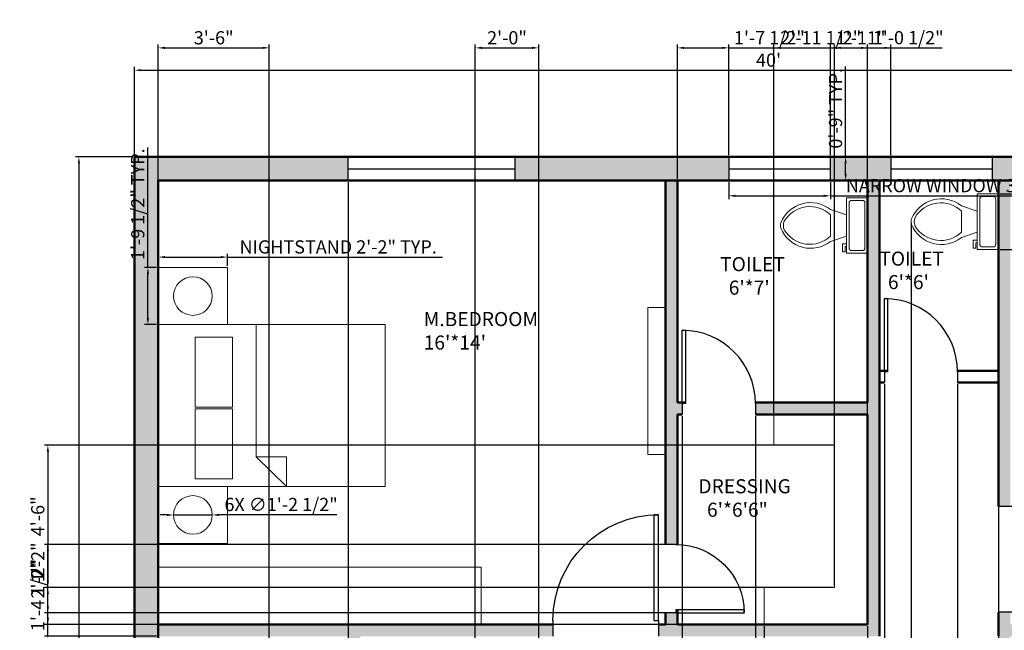
# Model space of a CAD drawing. Units: inches. Extents: x 2152 to 2718, y 1095 to 1798.
# Tile 4 of 5: x 2152 to 2524, y 1567 to 1798. Entities that reach past the tile are written whole.
import ezdxf

# ---------------------------------------------------------------- set-up
doc = ezdxf.new("R2010")
doc.units = ezdxf.units.IN
for name, color, linetype, lineweight in [('A-ANNO-DIMS', 130, 'Continuous', 18), ('A-AREA-IDEN', 130, 'Continuous', 25), ('A-FLOR-CASE', 10, 'Continuous', 20), ('A-FLOR-FIXT', 10, 'Continuous', 18), ('A-WALL-PATT', 210, 'Continuous', 13), ('DOOR', 160, 'Continuous', 25), ('FUR', 10, 'Continuous', 18), ('WALL', 7, 'Continuous', 50), ('WIND', 140, 'Continuous', 25)]:
    doc.layers.add(name, color=color, linetype=linetype, lineweight=lineweight)
doc.styles.get("Standard").update_dxf_attribs({"font": 'arial.ttf'})
doc.dimstyles.new('ISO-25', dxfattribs={"dimtxt": 5, "dimasz": 2.5, "dimexe": 1.25, "dimexo": 0.625, "dimtad": 1, "dimdec": 0, "dimlunit": 4, "dimtxsty": 'Standard', "dimcen": 2.5, "dimadec": 0, "dimazin": 0, "dimtfac": 1, "dimtdec": 0, "dimtmove": 0, "dimatfit": 3, "dimfxl": 1, "dimarcsym": 0})

# ---------------------------------------------------------------- blocks, each defined once
blk = doc.blocks.new('*U2')
for p, q in [((0, 0), (0, -6)), ((40, 0), (40, -6))]:
    blk.add_line(p, q)
blk.add_lwpolyline([(0, 0), (0, 40), (1.75, 40), (1.75, 0)], close=True)
blk.add_arc((0, 0), 40, 0, 90)
blk = doc.blocks.new('*U8')
for p, q in [((9.5, -6), (9.5, -2)), ((-10, -8.5), (-8, -8.5)), ((-10, -9.5), (-10, -8.5)), ((-7, -9.5), (-10, -9.5)), ((-8, -8.5), (-8, -8)), ((-7, -8), (-7, -9.5)), ((-4, -8), (-6, -14)), ((4, -8), (6, -14)), ((4, -14), (-4, -14))]:
    blk.add_line(p, q)
blk.add_lwpolyline([(10.5, -8), (10.5, 0), (-10.5, 0), (-10.5, -8)], close=True)
for points in [[(-9.5, -2), (-9.5, -6)], [(8.5, -1), (-8.5, -1)], [(-8.5, -7), (8.5, -7)]]:
    blk.add_lwpolyline(points)
for centre, radius, start, end in [((-8.62, -1.88), 0.884, 81.8699, 188.1301), ((8.62, -1.88), 0.884, 351.8699, 98.1301), ((-8.62, -6.12), 0.884, 171.8699, 278.1301), ((8.62, -6.12), 0.884, 261.8699, 8.1301), ((3.52, -21.58), 12.17, 141.4691, 247.9714), ((4.2, -21.82), 11.33, 136.3677, 238.9468), ((-3.52, -21.58), 12.17, 292.0284, 38.5307), ((-4.2, -21.82), 11.33, 301.053, 43.6321), ((0, -27.88), 4, 245.7318, 294.2682), ((0, -29), 4, 254.8605, 285.1395)]:
    blk.add_arc(centre, radius, start, end)
blk = doc.blocks.new('*D13')
at = {"layer": 'A-ANNO-DIMS', "color": 0, "lineweight": -2, "transparency": 16777216}
for p, q in [((2195.06, 1746.99), (2195.06, 1780.4)), ((2197.56, 1779.15), (2672.56, 1779.15)), ((2675.06, 1746.99), (2675.06, 1780.4))]:
    blk.add_line(p, q, dxfattribs=at)
at = {"layer": 'A-ANNO-DIMS', "color": 0, "transparency": 16777216}
for points in [[(2197.56, 1779.57), (2197.56, 1778.74), (2195.06, 1779.15)], [(2672.56, 1779.57), (2672.56, 1778.74), (2675.06, 1779.15)]]:
    blk.add_solid(points, dxfattribs=at)
at = {"layer": 'Defpoints', "color": 0, "transparency": 16777216}
for p in [(2675.06, 1779.15), (2195.06, 1746.37), (2675.06, 1746.37)]:
    blk.add_point(p, dxfattribs=at)
at = {"layer": 'A-ANNO-DIMS', "color": 0, "transparency": 16777216, "insert": (2435.06, 1782.33), "char_height": 5, "attachment_point": 5}
blk.add_mtext("40'", dxfattribs=at)
blk = doc.blocks.new('*D14')
at = {"layer": 'A-ANNO-DIMS', "color": 0, "lineweight": -2, "transparency": 16777216}
for p, q in [((2194.43, 1746.37), (2172.77, 1746.37)), ((2174.02, 1743.87), (2174.02, 1136.72)), ((2194.43, 1134.22), (2172.77, 1134.22))]:
    blk.add_line(p, q, dxfattribs=at)
at = {"layer": 'A-ANNO-DIMS', "color": 0, "transparency": 16777216}
for points in [[(2173.6, 1743.87), (2174.43, 1743.87), (2174.02, 1746.37)], [(2173.6, 1136.72), (2174.43, 1136.72), (2174.02, 1134.22)]]:
    blk.add_solid(points, dxfattribs=at)
at = {"layer": 'Defpoints', "color": 0, "transparency": 16777216}
for p in [(2195.06, 1746.37), (2174.02, 1134.22), (2195.06, 1134.22)]:
    blk.add_point(p, dxfattribs=at)
at = {"layer": 'A-ANNO-DIMS', "color": 0, "transparency": 16777216, "insert": (2170.84, 1440.29), "char_height": 5, "attachment_point": 5, "rotation": 90}
blk.add_mtext("51'", dxfattribs=at)
blk = doc.blocks.new('WIN-WIDE')
blk.add_line((0, 4.5), (63.07, 4.5))
blk.add_lwpolyline([(0, 9), (63.07, 9), (63.07, 0), (0, 0)], close=True)
blk = doc.blocks.new('WIN-NARROW')
blk.add_line((0, 4.5), (38.45, 4.5))
blk.add_lwpolyline([(0, 0), (38.45, 0), (38.45, 9), (0, 9)], close=True)
blk = doc.blocks.new('BED-DOUBLE')
for p, q in [((37.05, 61.24), (37.05, 11.23)), ((37.05, 11.23), (48.59, 11.23)), ((48.59, 0), (37.05, 11.23)), ((48.59, 11.23), (48.59, 0))]:
    blk.add_line(p, q)
for points in [[(0, 61.24), (85.82, 61.24), (85.82, 0), (0, 0)], [(13.94, 29.93), (28.11, 29.93), (28.11, 56.53), (13.94, 56.53)], [(13.94, 2.81), (28.11, 2.81), (28.11, 29.41), (13.94, 29.41)]]:
    blk.add_lwpolyline(points, close=True)
blk = doc.blocks.new('NIGHTSTAND')
blk.add_lwpolyline([(0, 21.63), (26.19, 21.63), (26.19, 0), (0, 0)], close=True)
blk.add_circle((13.1, 10.82), 7.32)
blk = doc.blocks.new('*D22')
at = {"layer": 'A-ANNO-DIMS', "color": 0, "lineweight": -2, "transparency": 16777216}
for p, q in [((2204.06, 1705.1), (2204.06, 1709.65)), ((2206.56, 1708.4), (2227.75, 1708.4)), ((2230.25, 1705.1), (2230.25, 1709.65)), ((2230.25, 1708.4), (2311.58, 1708.4))]:
    blk.add_line(p, q, dxfattribs=at)
at = {"layer": 'A-ANNO-DIMS', "color": 0, "transparency": 16777216}
for points in [[(2206.56, 1708.82), (2206.56, 1707.99), (2204.06, 1708.4)], [(2227.75, 1708.82), (2227.75, 1707.99), (2230.25, 1708.4)]]:
    blk.add_solid(points, dxfattribs=at)
at = {"layer": 'Defpoints', "color": 0, "transparency": 16777216}
for p in [(2230.25, 1708.4), (2204.06, 1704.48), (2230.25, 1704.48)]:
    blk.add_point(p, dxfattribs=at)
at = {"layer": 'A-ANNO-DIMS', "color": 0, "transparency": 16777216, "insert": (2272.16, 1711.61), "char_height": 5, "attachment_point": 5}
blk.add_mtext('NIGHTSTAND 2\'-2" TYP.', dxfattribs=at)
blk = doc.blocks.new('*D23')
at = {"layer": 'A-ANNO-DIMS', "color": 0, "lineweight": -2, "transparency": 16777216}
for p, q in [((2200.13, 1704.48), (2200.13, 1749.88)), ((2203.43, 1704.48), (2198.88, 1704.48)), ((2200.13, 1685.34), (2200.13, 1701.98)), ((2203.43, 1682.84), (2198.88, 1682.84))]:
    blk.add_line(p, q, dxfattribs=at)
at = {"layer": 'A-ANNO-DIMS', "color": 0, "transparency": 16777216}
for points in [[(2199.71, 1701.98), (2200.55, 1701.98), (2200.13, 1704.48)], [(2199.71, 1685.34), (2200.55, 1685.34), (2200.13, 1682.84)]]:
    blk.add_solid(points, dxfattribs=at)
at = {"layer": 'Defpoints', "color": 0, "transparency": 16777216}
for p in [(2200.13, 1704.48), (2204.06, 1704.48), (2204.06, 1682.84)]:
    blk.add_point(p, dxfattribs=at)
at = {"layer": 'A-ANNO-DIMS', "color": 0, "transparency": 16777216, "insert": (2196.92, 1728.43), "char_height": 5, "attachment_point": 5, "rotation": 90}
blk.add_mtext('1\'-9 1/2" TYP.', dxfattribs=at)
blk = doc.blocks.new('*D26')
at = {"layer": 'A-ANNO-DIMS', "color": 0, "lineweight": -2, "transparency": 16777216}
for p, q in [((2420.03, 1736.74), (2420.03, 1730.35)), ((2458.48, 1736.74), (2458.48, 1730.35)), ((2422.53, 1731.6), (2455.98, 1731.6)), ((2458.48, 1731.6), (2570.46, 1731.6))]:
    blk.add_line(p, q, dxfattribs=at)
at = {"layer": 'A-ANNO-DIMS', "color": 0, "transparency": 16777216}
for points in [[(2422.53, 1732.02), (2422.53, 1731.18), (2420.03, 1731.6)], [(2455.98, 1732.02), (2455.98, 1731.18), (2458.48, 1731.6)]]:
    blk.add_solid(points, dxfattribs=at)
at = {"layer": 'Defpoints', "color": 0, "transparency": 16777216}
for p in [(2420.03, 1737.37), (2458.48, 1737.37), (2458.48, 1731.6)]:
    blk.add_point(p, dxfattribs=at)
at = {"layer": 'A-ANNO-DIMS', "color": 0, "transparency": 16777216, "insert": (2515.72, 1734.81), "char_height": 5, "attachment_point": 5}
blk.add_mtext('NARROW WINDOW 3\'-2 1/2" TYP.', dxfattribs=at)
blk = doc.blocks.new('*D27')
at = {"layer": 'A-ANNO-DIMS', "color": 0, "lineweight": -2, "transparency": 16777216}
for p, q in [((2464.24, 1746.37), (2464.24, 1780.59)), ((2459.1, 1746.37), (2465.49, 1746.37)), ((2464.24, 1739.87), (2464.24, 1743.87)), ((2459.1, 1737.37), (2465.49, 1737.37))]:
    blk.add_line(p, q, dxfattribs=at)
at = {"layer": 'A-ANNO-DIMS', "color": 0, "transparency": 16777216}
for points in [[(2463.83, 1743.87), (2464.66, 1743.87), (2464.24, 1746.37)], [(2463.83, 1739.87), (2464.66, 1739.87), (2464.24, 1737.37)]]:
    blk.add_solid(points, dxfattribs=at)
at = {"layer": 'Defpoints', "color": 0, "transparency": 16777216}
for p in [(2458.48, 1746.37), (2464.24, 1746.37), (2458.48, 1737.37)]:
    blk.add_point(p, dxfattribs=at)
at = {"layer": 'A-ANNO-DIMS', "color": 0, "transparency": 16777216, "insert": (2461.07, 1764.73), "char_height": 5, "attachment_point": 5, "rotation": 90}
blk.add_mtext('0\'-9" TYP.', dxfattribs=at)
blk = doc.blocks.new('*D36')
at = {"layer": 'A-ANNO-DIMS', "color": 0, "lineweight": -2, "transparency": 16777216}
for p, q in [((2204.06, 1736.74), (2204.06, 1098.09)), ((2275.93, 1736.74), (2275.93, 1098.09)), ((2206.56, 1099.34), (2273.43, 1099.34))]:
    blk.add_line(p, q, dxfattribs=at)
at = {"layer": 'A-ANNO-DIMS', "color": 0, "transparency": 16777216}
for points in [[(2206.56, 1099.75), (2206.56, 1098.92), (2204.06, 1099.34)], [(2273.43, 1099.75), (2273.43, 1098.92), (2275.93, 1099.34)]]:
    blk.add_solid(points, dxfattribs=at)
at = {"layer": 'Defpoints', "color": 0, "transparency": 16777216}
for p in [(2204.06, 1737.37), (2275.93, 1737.37), (2275.93, 1099.34)]:
    blk.add_point(p, dxfattribs=at)
at = {"layer": 'A-ANNO-DIMS', "color": 0, "transparency": 16777216, "insert": (2240, 1102.51), "char_height": 5, "attachment_point": 5}
blk.add_mtext('6\'-0"', dxfattribs=at)
blk = doc.blocks.new('*D37')
at = {"layer": 'A-ANNO-DIMS', "color": 0, "lineweight": -2, "transparency": 16777216}
for p, q in [((2400.56, 1737.99), (2400.56, 1788.86)), ((2403.06, 1787.61), (2417.53, 1787.61)), ((2420.03, 1746.99), (2420.03, 1788.86)), ((2420.03, 1787.61), (2448.25, 1787.61))]:
    blk.add_line(p, q, dxfattribs=at)
at = {"layer": 'A-ANNO-DIMS', "color": 0, "transparency": 16777216}
for points in [[(2403.06, 1788.03), (2403.06, 1787.19), (2400.56, 1787.61)], [(2417.53, 1788.03), (2417.53, 1787.19), (2420.03, 1787.61)]]:
    blk.add_solid(points, dxfattribs=at)
at = {"layer": 'Defpoints', "color": 0, "transparency": 16777216}
for p in [(2420.03, 1787.61), (2420.03, 1746.37), (2400.56, 1737.37)]:
    blk.add_point(p, dxfattribs=at)
at = {"layer": 'A-ANNO-DIMS', "color": 0, "transparency": 16777216, "insert": (2435.39, 1790.82), "char_height": 5, "attachment_point": 5}
blk.add_mtext('1\'-7 1/2"', dxfattribs=at)
blk = doc.blocks.new('*D38')
at = {"layer": 'A-ANNO-DIMS', "color": 0, "lineweight": -2, "transparency": 16777216}
for p, q in [((2458.48, 1746.99), (2458.48, 1788.86)), ((2460.98, 1787.61), (2478.85, 1787.61)), ((2481.35, 1746.99), (2481.35, 1788.86))]:
    blk.add_line(p, q, dxfattribs=at)
at = {"layer": 'A-ANNO-DIMS', "color": 0, "transparency": 16777216}
for points in [[(2460.98, 1788.03), (2460.98, 1787.19), (2458.48, 1787.61)], [(2478.85, 1788.03), (2478.85, 1787.19), (2481.35, 1787.61)]]:
    blk.add_solid(points, dxfattribs=at)
at = {"layer": 'Defpoints', "color": 0, "transparency": 16777216}
for p in [(2481.35, 1787.61), (2458.48, 1746.37), (2481.35, 1746.37)]:
    blk.add_point(p, dxfattribs=at)
at = {"layer": 'A-ANNO-DIMS', "color": 0, "transparency": 16777216, "insert": (2469.91, 1790.75), "char_height": 5, "attachment_point": 5}
blk.add_mtext('1\'-11"', dxfattribs=at)
blk = doc.blocks.new('*D40')
at = {"layer": 'A-ANNO-DIMS', "color": 0, "lineweight": -2, "transparency": 16777216}
for p, q in [((2162.26, 1564.87), (2162.26, 1593.09)), ((2203.43, 1564.87), (2161.01, 1564.87)), ((2162.26, 1550.66), (2162.26, 1562.37)), ((2203.43, 1548.16), (2161.01, 1548.16))]:
    blk.add_line(p, q, dxfattribs=at)
at = {"layer": 'A-ANNO-DIMS', "color": 0, "transparency": 16777216}
for points in [[(2161.84, 1562.37), (2162.68, 1562.37), (2162.26, 1564.87)], [(2161.84, 1550.66), (2162.68, 1550.66), (2162.26, 1548.16)]]:
    blk.add_solid(points, dxfattribs=at)
at = {"layer": 'Defpoints', "color": 0, "transparency": 16777216}
for p in [(2162.26, 1564.87), (2204.06, 1564.87), (2204.06, 1548.16)]:
    blk.add_point(p, dxfattribs=at)
at = {"layer": 'A-ANNO-DIMS', "color": 0, "transparency": 16777216, "insert": (2159.05, 1580.23), "char_height": 5, "attachment_point": 5, "rotation": 90}
blk.add_mtext('1\'-4 1/2"', dxfattribs=at)
blk = doc.blocks.new('*D42')
at = {"layer": 'A-ANNO-DIMS', "color": 0, "lineweight": -2, "transparency": 16777216}
for p, q in [((2204.06, 1176.99), (2204.06, 1788.86)), ((2206.56, 1787.61), (2243.52, 1787.61)), ((2246.02, 1176.99), (2246.02, 1788.86))]:
    blk.add_line(p, q, dxfattribs=at)
at = {"layer": 'A-ANNO-DIMS', "color": 0, "transparency": 16777216}
for points in [[(2206.56, 1788.03), (2206.56, 1787.19), (2204.06, 1787.61)], [(2243.52, 1788.03), (2243.52, 1787.19), (2246.02, 1787.61)]]:
    blk.add_solid(points, dxfattribs=at)
at = {"layer": 'Defpoints', "color": 0, "transparency": 16777216}
for p in [(2246.02, 1787.61), (2204.06, 1176.37), (2246.02, 1176.37)]:
    blk.add_point(p, dxfattribs=at)
at = {"layer": 'A-ANNO-DIMS', "color": 0, "transparency": 16777216, "insert": (2225.04, 1790.79), "char_height": 5, "attachment_point": 5}
blk.add_mtext('3\'-6"', dxfattribs=at)
blk = doc.blocks.new('*D50')
at = {"layer": 'A-ANNO-DIMS', "color": 0, "lineweight": -2, "transparency": 16777216}
for p, q in [((2707.86, 1560.98), (2707.86, 1589.76)), ((2281.18, 1560.98), (2709.11, 1560.98)), ((2707.86, 1539.09), (2707.86, 1558.48)), ((2281.18, 1536.59), (2709.11, 1536.59))]:
    blk.add_line(p, q, dxfattribs=at)
at = {"layer": 'A-ANNO-DIMS', "color": 0, "transparency": 16777216}
for points in [[(2707.44, 1558.48), (2708.28, 1558.48), (2707.86, 1560.98)], [(2707.44, 1539.09), (2708.28, 1539.09), (2707.86, 1536.59)]]:
    blk.add_solid(points, dxfattribs=at)
at = {"layer": 'Defpoints', "color": 0, "transparency": 16777216}
for p in [(2280.56, 1560.98), (2707.86, 1560.98), (2280.56, 1536.59)]:
    blk.add_point(p, dxfattribs=at)
at = {"layer": 'A-ANNO-DIMS', "color": 0, "transparency": 16777216, "insert": (2704.65, 1576.62), "char_height": 5, "attachment_point": 5, "rotation": 90}
blk.add_mtext('2\'-0 1/2"', dxfattribs=at)
blk = doc.blocks.new('*D51')
at = {"layer": 'A-ANNO-DIMS', "color": 0, "lineweight": -2, "transparency": 16777216}
for p, q in [((2399.93, 1599.6), (2161.01, 1599.6)), ((2162.26, 1576.22), (2162.26, 1597.1)), ((2399.32, 1573.72), (2161.01, 1573.72))]:
    blk.add_line(p, q, dxfattribs=at)
at = {"layer": 'A-ANNO-DIMS', "color": 0, "transparency": 16777216}
for points in [[(2161.84, 1597.1), (2162.68, 1597.1), (2162.26, 1599.6)], [(2161.84, 1576.22), (2162.68, 1576.22), (2162.26, 1573.72)]]:
    blk.add_solid(points, dxfattribs=at)
at = {"layer": 'Defpoints', "color": 0, "transparency": 16777216}
for p in [(2162.26, 1599.6), (2400.56, 1599.6), (2399.94, 1573.72)]:
    blk.add_point(p, dxfattribs=at)
at = {"layer": 'A-ANNO-DIMS', "color": 0, "transparency": 16777216, "insert": (2159.12, 1586.66), "char_height": 5, "attachment_point": 5, "rotation": 90}
blk.add_mtext('2\'-2"', dxfattribs=at)
blk = doc.blocks.new('*D52')
at = {"layer": 'A-ANNO-DIMS', "color": 0, "lineweight": -2, "transparency": 16777216}
for p, q in [((2402.42, 1648.24), (2402.42, 1098.09)), ((2430.09, 1648.24), (2430.09, 1098.09)), ((2404.92, 1099.34), (2427.59, 1099.34))]:
    blk.add_line(p, q, dxfattribs=at)
at = {"layer": 'A-ANNO-DIMS', "color": 0, "transparency": 16777216}
for points in [[(2404.92, 1099.75), (2404.92, 1098.92), (2402.42, 1099.34)], [(2427.59, 1099.75), (2427.59, 1098.92), (2430.09, 1099.34)]]:
    blk.add_solid(points, dxfattribs=at)
at = {"layer": 'Defpoints', "color": 0, "transparency": 16777216}
for p in [(2402.42, 1648.87), (2430.09, 1648.87), (2430.09, 1099.34)]:
    blk.add_point(p, dxfattribs=at)
at = {"layer": 'A-ANNO-DIMS', "color": 0, "transparency": 16777216, "insert": (2416.26, 1102.55), "char_height": 5, "attachment_point": 5}
blk.add_mtext('2\'-3 1/2"', dxfattribs=at)
blk = doc.blocks.new('*D57')
at = {"layer": 'A-ANNO-DIMS', "color": 0, "lineweight": -2, "transparency": 16777216}
for p, q in [((2489.06, 1721.19), (2489.06, 1098.09)), ((2522.06, 1710.69), (2522.06, 1098.09)), ((2491.56, 1099.34), (2519.56, 1099.34))]:
    blk.add_line(p, q, dxfattribs=at)
at = {"layer": 'A-ANNO-DIMS', "color": 0, "transparency": 16777216}
for points in [[(2491.56, 1099.75), (2491.56, 1098.92), (2489.06, 1099.34)], [(2519.56, 1099.75), (2519.56, 1098.92), (2522.06, 1099.34)]]:
    blk.add_solid(points, dxfattribs=at)
at = {"layer": 'Defpoints', "color": 0, "transparency": 16777216}
for p in [(2489.06, 1721.81), (2522.06, 1711.31), (2522.06, 1099.34)]:
    blk.add_point(p, dxfattribs=at)
at = {"layer": 'A-ANNO-DIMS', "color": 0, "transparency": 16777216, "insert": (2505.56, 1102.51), "char_height": 5, "attachment_point": 5}
blk.add_mtext('2\'-9"', dxfattribs=at)
blk = doc.blocks.new('*D58')
at = {"layer": 'A-ANNO-DIMS', "color": 0, "lineweight": -2, "transparency": 16777216}
for p, q in [((2522.68, 1732.31), (2709.11, 1732.31)), ((2707.86, 1729.81), (2707.86, 1713.81)), ((2522.68, 1711.31), (2709.11, 1711.31))]:
    blk.add_line(p, q, dxfattribs=at)
at = {"layer": 'A-ANNO-DIMS', "color": 0, "transparency": 16777216}
for points in [[(2707.44, 1729.81), (2708.28, 1729.81), (2707.86, 1732.31)], [(2707.44, 1713.81), (2708.28, 1713.81), (2707.86, 1711.31)]]:
    blk.add_solid(points, dxfattribs=at)
at = {"layer": 'Defpoints', "color": 0, "transparency": 16777216}
for p in [(2522.06, 1732.31), (2522.06, 1711.31), (2707.86, 1711.31)]:
    blk.add_point(p, dxfattribs=at)
at = {"layer": 'A-ANNO-DIMS', "color": 0, "transparency": 16777216, "insert": (2704.68, 1721.81), "char_height": 5, "attachment_point": 5, "rotation": 90}
blk.add_mtext('1\'-9"', dxfattribs=at)
blk = doc.blocks.new('*D59')
at = {"layer": 'A-ANNO-DIMS', "color": 0, "lineweight": -2, "transparency": 16777216}
for p, q in [((2478.92, 1660.24), (2478.92, 1098.09)), ((2506.58, 1660.24), (2506.58, 1098.09)), ((2481.42, 1099.34), (2504.08, 1099.34))]:
    blk.add_line(p, q, dxfattribs=at)
at = {"layer": 'A-ANNO-DIMS', "color": 0, "transparency": 16777216}
for points in [[(2481.42, 1099.75), (2481.42, 1098.92), (2478.92, 1099.34)], [(2504.08, 1099.75), (2504.08, 1098.92), (2506.58, 1099.34)]]:
    blk.add_solid(points, dxfattribs=at)
at = {"layer": 'Defpoints', "color": 0, "transparency": 16777216}
for p in [(2478.92, 1660.87), (2506.58, 1660.87), (2506.58, 1099.34)]:
    blk.add_point(p, dxfattribs=at)
at = {"layer": 'A-ANNO-DIMS', "color": 0, "transparency": 16777216, "insert": (2492.75, 1102.55), "char_height": 5, "attachment_point": 5}
blk.add_mtext('2\'-3 1/2"', dxfattribs=at)
blk = doc.blocks.new('*D60')
at = {"layer": 'A-ANNO-DIMS', "color": 0, "lineweight": -2, "transparency": 16777216}
for p, q in [((2433.42, 1568.74), (2433.42, 1098.09)), ((2472.56, 1568.74), (2472.56, 1098.09)), ((2435.92, 1099.34), (2470.06, 1099.34))]:
    blk.add_line(p, q, dxfattribs=at)
at = {"layer": 'A-ANNO-DIMS', "color": 0, "transparency": 16777216}
for points in [[(2435.92, 1099.75), (2435.92, 1098.92), (2433.42, 1099.34)], [(2470.06, 1099.75), (2470.06, 1098.92), (2472.56, 1099.34)]]:
    blk.add_solid(points, dxfattribs=at)
at = {"layer": 'Defpoints', "color": 0, "transparency": 16777216}
for p in [(2433.42, 1569.37), (2472.56, 1569.37), (2472.56, 1099.34)]:
    blk.add_point(p, dxfattribs=at)
at = {"layer": 'A-ANNO-DIMS', "color": 0, "transparency": 16777216, "insert": (2452.99, 1102.51), "char_height": 5, "attachment_point": 5}
blk.add_mtext('3\'-3"', dxfattribs=at)
blk = doc.blocks.new('*D61')
at = {"layer": 'A-ANNO-DIMS', "color": 0, "lineweight": -2, "transparency": 16777216}
for p, q in [((2437.12, 1649.49), (2437.12, 1788.86)), ((2439.62, 1787.61), (2470.06, 1787.61)), ((2472.56, 1649.49), (2472.56, 1788.86))]:
    blk.add_line(p, q, dxfattribs=at)
at = {"layer": 'A-ANNO-DIMS', "color": 0, "transparency": 16777216}
for points in [[(2439.62, 1788.03), (2439.62, 1787.19), (2437.12, 1787.61)], [(2470.06, 1788.03), (2470.06, 1787.19), (2472.56, 1787.61)]]:
    blk.add_solid(points, dxfattribs=at)
at = {"layer": 'Defpoints', "color": 0, "transparency": 16777216}
for p in [(2472.56, 1787.61), (2437.12, 1648.87), (2472.56, 1648.87)]:
    blk.add_point(p, dxfattribs=at)
at = {"layer": 'A-ANNO-DIMS', "color": 0, "transparency": 16777216, "insert": (2454.84, 1790.82), "char_height": 5, "attachment_point": 5}
blk.add_mtext('2\'-11 1/2"', dxfattribs=at)
blk = doc.blocks.new('*D62')
at = {"layer": 'A-ANNO-DIMS', "color": 0, "lineweight": -2, "transparency": 16777216}
for p, q in [((2459.4, 1637.23), (2161.01, 1637.23)), ((2162.26, 1634.73), (2162.26, 1585.82)), ((2459.4, 1583.32), (2161.01, 1583.32))]:
    blk.add_line(p, q, dxfattribs=at)
at = {"layer": 'A-ANNO-DIMS', "color": 0, "transparency": 16777216}
for points in [[(2161.84, 1634.73), (2162.68, 1634.73), (2162.26, 1637.23)], [(2161.84, 1585.82), (2162.68, 1585.82), (2162.26, 1583.32)]]:
    blk.add_solid(points, dxfattribs=at)
at = {"layer": 'Defpoints', "color": 0, "transparency": 16777216}
for p in [(2460.02, 1637.23), (2162.26, 1583.32), (2460.02, 1583.32)]:
    blk.add_point(p, dxfattribs=at)
at = {"layer": 'A-ANNO-DIMS', "color": 0, "transparency": 16777216, "insert": (2159.08, 1610.28), "char_height": 5, "attachment_point": 5, "rotation": 90}
blk.add_mtext('4\'-6"', dxfattribs=at)
blk = doc.blocks.new('*D63')
at = {"layer": 'A-ANNO-DIMS', "color": 0, "lineweight": -2, "transparency": 16777216}
for p, q in [((2460.02, 1583.95), (2460.02, 1788.86)), ((2462.52, 1787.61), (2470.06, 1787.61)), ((2472.56, 1569.99), (2472.56, 1788.86)), ((2472.56, 1787.61), (2500.78, 1787.61))]:
    blk.add_line(p, q, dxfattribs=at)
at = {"layer": 'A-ANNO-DIMS', "color": 0, "transparency": 16777216}
for points in [[(2462.52, 1788.03), (2462.52, 1787.19), (2460.02, 1787.61)], [(2470.06, 1788.03), (2470.06, 1787.19), (2472.56, 1787.61)]]:
    blk.add_solid(points, dxfattribs=at)
at = {"layer": 'Defpoints', "color": 0, "transparency": 16777216}
for p in [(2472.56, 1787.61), (2460.02, 1583.32), (2472.56, 1569.37)]:
    blk.add_point(p, dxfattribs=at)
at = {"layer": 'A-ANNO-DIMS', "color": 0, "transparency": 16777216, "insert": (2487.92, 1790.82), "char_height": 5, "attachment_point": 5}
blk.add_mtext('1\'-0 1/2"', dxfattribs=at)
blk = doc.blocks.new('*D64')
at = {"layer": 'A-ANNO-DIMS', "color": 0, "lineweight": -2, "transparency": 16777216}
for p, q in [((2162.26, 1583.32), (2162.26, 1599.9)), ((2432.79, 1583.32), (2161.01, 1583.32)), ((2162.26, 1571.87), (2162.26, 1580.82)), ((2432.79, 1569.37), (2161.01, 1569.37))]:
    blk.add_line(p, q, dxfattribs=at)
at = {"layer": 'A-ANNO-DIMS', "color": 0, "transparency": 16777216}
for points in [[(2161.84, 1580.82), (2162.68, 1580.82), (2162.26, 1583.32)], [(2161.84, 1571.87), (2162.68, 1571.87), (2162.26, 1569.37)]]:
    blk.add_solid(points, dxfattribs=at)
at = {"layer": 'Defpoints', "color": 0, "transparency": 16777216}
for p in [(2162.26, 1583.32), (2433.42, 1583.32), (2433.42, 1569.37)]:
    blk.add_point(p, dxfattribs=at)
at = {"layer": 'A-ANNO-DIMS', "color": 0, "transparency": 16777216, "insert": (2159.12, 1592.86), "char_height": 5, "attachment_point": 5, "rotation": 90}
blk.add_mtext('1\'-2"', dxfattribs=at)
blk = doc.blocks.new('*D68')
at = {"layer": 'A-ANNO-DIMS', "color": 0, "lineweight": -2, "transparency": 16777216}
for p, q in [((2324.06, 1258.93), (2324.06, 1788.86)), ((2326.56, 1787.61), (2345.56, 1787.61)), ((2348.06, 1258.93), (2348.06, 1788.86))]:
    blk.add_line(p, q, dxfattribs=at)
at = {"layer": 'A-ANNO-DIMS', "color": 0, "transparency": 16777216}
for points in [[(2326.56, 1788.03), (2326.56, 1787.19), (2324.06, 1787.61)], [(2345.56, 1788.03), (2345.56, 1787.19), (2348.06, 1787.61)]]:
    blk.add_solid(points, dxfattribs=at)
at = {"layer": 'Defpoints', "color": 0, "transparency": 16777216}
for p in [(2348.06, 1787.61), (2324.06, 1258.3), (2348.06, 1258.3)]:
    blk.add_point(p, dxfattribs=at)
at = {"layer": 'A-ANNO-DIMS', "color": 0, "transparency": 16777216, "insert": (2336.06, 1790.79), "char_height": 5, "attachment_point": 5}
blk.add_mtext('2\'-0"', dxfattribs=at)
blk = doc.blocks.new('*D71')
at = {"layer": 'A-ANNO-DIMS', "color": 0, "lineweight": -2, "transparency": 16777216}
for p, q in [((2207.33, 1610.78), (2204.83, 1610.78)), ((2209.83, 1610.78), (2224.48, 1610.79)), ((2271.61, 1610.79), (2226.98, 1610.79))]:
    blk.add_line(p, q, dxfattribs=at)
at = {"layer": 'A-ANNO-DIMS', "color": 0, "transparency": 16777216}
for points in [[(2207.33, 1611.2), (2207.33, 1610.37), (2209.83, 1610.78)], [(2226.98, 1611.2), (2226.98, 1610.37), (2224.48, 1610.79)]]:
    blk.add_solid(points, dxfattribs=at)
at = {"layer": 'Defpoints', "color": 0, "transparency": 16777216}
for p in [(2209.83, 1610.78), (2224.48, 1610.79)]:
    blk.add_point(p, dxfattribs=at)
at = {"layer": 'A-ANNO-DIMS', "color": 0, "transparency": 16777216, "insert": (2250.54, 1614.1), "char_height": 5, "attachment_point": 5, "rotation": 0.0031}
blk.add_mtext('6X ∅1\'-2 1/2"', dxfattribs=at)

msp = doc.modelspace()

# ---------------------------------------------------------------- hatches: boundary and pattern name
at = {"layer": 'A-WALL-PATT'}
h = msp.add_hatch(color=256, dxfattribs=at)
h.dxf.hatch_style = 1
h.paths.add_polyline_path([(2204.06, 1737.37), (2275.93, 1737.37), (2275.93, 1746.37), (2195.06, 1746.37), (2195.06, 1548.16), (2204.06, 1548.16)])
h.paths.add_polyline_path([(2567.46, 1746.37), (2519.79, 1746.37), (2519.79, 1737.37), (2549.06, 1737.37), (2567.46, 1737.37)])
h.paths.add_polyline_path([(2526.56, 1706.63), (2526.56, 1737.37), (2522.06, 1737.37), (2522.06, 1614.04), (2526.56, 1614.04), (2526.56, 1660.87)])
h.paths.add_polyline_path([(2477.06, 1737.37), (2472.56, 1737.37), (2472.56, 1653.37), (2430.09, 1653.37), (2430.09, 1648.87), (2472.56, 1648.87), (2472.56, 1569.37), (2400.56, 1569.37), (2400.56, 1573.72), (2399.94, 1573.72), (2396.06, 1573.72), (2396.06, 1569.37), (2393.45, 1569.37), (2393.45, 1564.87), (2477.06, 1564.87), (2477.06, 1648.87)])
h.paths.add_polyline_path([(2400.56, 1737.37), (2396.06, 1737.37), (2396.06, 1599.61), (2400.56, 1599.61), (2400.56, 1648.87), (2402.42, 1648.87), (2402.42, 1653.37), (2400.56, 1653.37)], flags=17)
h.paths.add_polyline_path([(2353.45, 1569.37), (2204.06, 1569.37), (2204.06, 1564.87), (2353.45, 1564.87)])
h.paths.add_polyline_path([(2280.56, 1492.87), (2221.07, 1492.87), (2221.07, 1488.37), (2280.56, 1488.37)])
h.paths.add_polyline_path([(2221.07, 1492.87), (2204.06, 1492.87), (2204.06, 1488.37), (2221.07, 1488.37)])
h.paths.add_polyline_path([(2280.56, 1536.59), (2276.9, 1536.59, -0.008622), (2276.06, 1536.6), (2276.06, 1492.87), (2280.56, 1492.87)])
h.paths.add_polyline_path([(2280.56, 1564.87), (2276.06, 1564.87), (2276.06, 1560.98), (2276.9, 1560.98), (2280.56, 1560.98)])
h.paths.add_polyline_path([(2675.06, 1746.37), (2630.54, 1746.37), (2630.54, 1737.37), (2666.06, 1737.37), (2666.06, 1384.87), (2675.06, 1384.87)])
h.paths.add_polyline_path([(2666.06, 1569.37), (2578.28, 1569.37), (2526.56, 1569.37), (2526.56, 1574.04), (2522.06, 1574.04), (2522.06, 1564.87), (2522.06, 1560.6), (2526.56, 1560.6), (2526.56, 1564.87), (2666.06, 1564.87)])
h.paths.add_polyline_path([(2526.56, 1520.6), (2522.06, 1520.6), (2522.06, 1384.87), (2570.2, 1384.87), (2570.2, 1393.87), (2526.56, 1393.87)])
h.paths.add_polyline_path([(2666.06, 1393.87), (2633.28, 1393.87), (2633.28, 1384.87), (2666.06, 1384.87)], flags=17)
h.paths.add_polyline_path([(2522.06, 1393.87), (2306.06, 1393.87), (2280.56, 1393.87), (2280.56, 1384.87), (2301.56, 1384.87), (2522.06, 1384.87)])
h.paths.add_polyline_path([(2280.56, 1393.87), (2204.06, 1393.87), (2204.06, 1384.87), (2232.43, 1384.87), (2280.56, 1384.87)])
h.paths.add_polyline_path([(2204.06, 1509.71), (2195.06, 1509.71), (2195.06, 1364.72), (2204.06, 1364.72), (2204.06, 1384.87)])
h.paths.add_polyline_path([(2204.06, 1326.27), (2195.06, 1326.27), (2195.06, 1302.62), (2201.06, 1302.62), (2204.06, 1302.62), (2204.06, 1308.37)])
h.paths.add_polyline_path([(2280.56, 1384.87), (2276.06, 1384.87), (2276.06, 1312.87), (2273.63, 1312.87), (2273.63, 1312.11), (2273.63, 1308.37), (2280.56, 1308.37)])
h.paths.add_polyline_path([(2248.67, 1312.11, -0.007577), (2248.69, 1312.87), (2204.06, 1312.87), (2204.06, 1308.37), (2248.67, 1308.37)])
h.paths.add_polyline_path([(2364.43, 1297.87), (2364.43, 1300.87), (2357.06, 1300.87), (2357.06, 1291.87), (2364.43, 1291.87)])
h.paths.add_polyline_path([(2428.34, 1300.87), (2404.32, 1300.87, -0.01877), (2404.43, 1297.87), (2404.43, 1291.87), (2428.34, 1291.87)])
h.paths.add_polyline_path([(2522.06, 1384.87), (2513.06, 1384.87), (2513.06, 1300.87), (2491.42, 1300.87), (2491.42, 1291.87), (2522.06, 1291.87)])
h.paths.add_polyline_path([(2357.06, 1384.87), (2348.06, 1384.87), (2348.06, 1176.37), (2309.1, 1176.37), (2309.1, 1167.37), (2357.06, 1167.37), (2357.06, 1173.65)])
h.paths.add_polyline_path([(2475.5, 1693.24), (2504.24, 1693.24), (2504.24, 1713.14), (2475.5, 1713.14)], flags=9)
h = msp.add_hatch(color=256, dxfattribs=at)
h.dxf.hatch_style = 1
h.paths.add_polyline_path([(2420.03, 1746.37), (2339.01, 1746.37), (2339.01, 1737.37), (2396.06, 1737.37), (2420.03, 1737.37)])
h.paths.add_polyline_path([(2481.35, 1746.37), (2458.48, 1746.37), (2458.48, 1737.37), (2472.56, 1737.37), (2481.35, 1737.37)])

# ---------------------------------------------------------------- linework, layer by layer
at = {"layer": 'A-FLOR-CASE'}
for p, q in [((2437.12, 1648.87), (2437.12, 1637.23)), ((2437.12, 1637.23), (2460.02, 1637.23)), ((2460.02, 1637.23), (2460.02, 1583.32)), ((2460.02, 1583.32), (2433.42, 1583.32)), ((2433.42, 1583.32), (2433.42, 1569.37))]:
    msp.add_line(p, q, dxfattribs=at)
for points in [[(2396.06, 1689.26), (2389.32, 1689.26), (2389.32, 1633.69), (2396.06, 1633.69)], [(2204.06, 1569.37), (2326.3, 1569.37), (2326.3, 1590.98), (2204.06, 1590.98)]]:
    msp.add_lwpolyline(points, close=True, dxfattribs=at)
at = {"layer": 'WALL'}
for p, q in [((2195.06, 1746.37), (2675.06, 1746.37)), ((2195.06, 1302.62), (2195.06, 1746.37)), ((2204.06, 1737.37), (2666.06, 1737.37)), ((2204.06, 1737.37), (2396.06, 1737.37)), ((2204.06, 1300.87), (2204.06, 1737.37)), ((2396.06, 1737.37), (2396.06, 1599.61)), ((2400.56, 1737.37), (2400.56, 1653.37)), ((2400.56, 1737.37), (2472.56, 1737.37)), ((2472.56, 1737.37), (2472.56, 1653.37)), ((2477.06, 1737.37), (2477.06, 1648.87)), ((2477.06, 1737.37), (2549.06, 1737.37)), ((2522.06, 1737.37), (2522.06, 1665.37)), ((2522.06, 1737.37), (2522.06, 1614.04)), ((2480.13, 1665.37), (2477.06, 1665.37)), ((2522.06, 1665.37), (2506.58, 1665.37)), ((2478.92, 1660.87), (2477.06, 1660.87)), ((2522.06, 1660.87), (2506.58, 1660.87)), ((2403.63, 1653.37), (2400.56, 1653.37)), ((2472.56, 1653.37), (2430.08, 1653.37)), ((2400.56, 1648.87), (2400.56, 1599.6)), ((2402.42, 1648.87), (2400.56, 1648.87)), ((2472.56, 1648.87), (2430.09, 1648.87)), ((2472.56, 1648.87), (2472.56, 1569.37)), ((2477.06, 1648.87), (2477.06, 1564.87)), ((2396.06, 1573.72), (2396.06, 1569.37)), ((2400.56, 1574.85), (2400.56, 1569.37)), ((2522.06, 1574.04), (2522.06, 1564.87)), ((2353.45, 1569.37), (2204.06, 1569.37)), ((2396.06, 1569.37), (2393.45, 1569.37)), ((2472.56, 1569.37), (2400.56, 1569.37))]:
    msp.add_line(p, q, dxfattribs=at)

# ---------------------------------------------------------------- block references
at = {"layer": 'A-FLOR-FIXT', "xscale": -1, "rotation": 270}
for p in [(2472.56, 1720.37), (2522.06, 1721.81)]:
    msp.add_blockref('*U8', p, dxfattribs=at)
at = {"layer": 'DOOR', "xscale": 0.691524538410026, "yscale": 0.691524538410026, "zscale": 0.691524538410026}
for p in [(2478.92, 1665.02), (2402.42, 1653.02)]:
    msp.add_blockref('*U2', p, dxfattribs=at)
at = {"layer": 'DOOR', "xscale": -1, "rotation": 270}
msp.add_blockref('*U2', (2528.06, 1574.04), dxfattribs=at)
at = {"layer": 'DOOR', "xscale": -1}
msp.add_blockref('*U2', (2393.45, 1570.87), dxfattribs=at)
at = {"layer": 'DOOR', "xscale": -0.6472126286789514, "yscale": 0.6472126286789514, "zscale": 0.6472126286789514, "rotation": 270}
msp.add_blockref('*U2', (2399.94, 1573.72), dxfattribs=at)
at = {"layer": 'FUR'}
for name, p in [('NIGHTSTAND', (2204.06, 1682.84)), ('BED-DOUBLE', (2204.06, 1621.6)), ('NIGHTSTAND', (2204.06, 1599.97))]:
    msp.add_blockref(name, p, dxfattribs=at)
at = {"layer": 'WIND'}
for name, p in [('WIN-WIDE', (2275.93, 1737.37)), ('WIN-NARROW', (2420.03, 1737.37)), ('WIN-NARROW', (2481.35, 1737.37))]:
    msp.add_blockref(name, p, dxfattribs=at)

# ---------------------------------------------------------------- texts
at = {"layer": 'A-AREA-IDEN', "char_height": 5.331, "attachment_point": 1}
for s, insert in [("TOILET\\P  6'*7'", (2416.74, 1708.4)), ("TOILET\\P  6'*6'", (2477.01, 1710.49)), ("M.BEDROOM\\P16'*14'", (2304.52, 1687.61)), ('DRESSING\\P  6\'*6\'6"', (2408.51, 1624.31))]:
    msp.add_mtext_dynamic_manual_height_columns(s, width=138.497, gutter_width=26.66, heights=[0], dxfattribs=dict(at, insert=insert))

# ---------------------------------------------------------------- dimensions: what is measured, and where the dimension line sits
at = {"layer": 'A-ANNO-DIMS'}
for base, p1, p2, override, picture, middle in [((2420.03, 1787.61), (2400.56, 1737.37), (2420.03, 1746.37), {"dimdec": 1, "dimlfac": 1, "dimrnd": 0, "dimzin": 1, "dimdsep": 46, "dimlunit": 4, "dimfrac": 2}, '*D37', (2435.39, 1790.82)), ((2472.56, 1787.61), (2437.12, 1648.87), (2472.56, 1648.87), {"dimdec": 1, "dimlfac": 1, "dimrnd": 0, "dimzin": 1, "dimdsep": 46, "dimlunit": 4, "dimfrac": 2}, '*D61', (2454.84, 1790.82)), ((2472.56, 1787.61), (2460.02, 1583.32), (2472.56, 1569.37), {"dimdec": 1, "dimlfac": 1, "dimrnd": 0, "dimzin": 1, "dimdsep": 46, "dimlunit": 4, "dimfrac": 2}, '*D63', (2487.92, 1790.82)), ((2246.02, 1787.61), (2204.06, 1176.37), (2246.02, 1176.37), {"dimdec": 1, "dimlfac": 1, "dimrnd": 0, "dimzin": 1, "dimdsep": 46, "dimlunit": 4, "dimfrac": 2}, '*D42', (2225.04, 1790.79)), ((2348.06, 1787.61), (2324.06, 1258.3), (2348.06, 1258.3), {"dimdec": 1, "dimlfac": 1, "dimrnd": 0, "dimzin": 1, "dimdsep": 46, "dimlunit": 4, "dimfrac": 2}, '*D68', (2336.06, 1790.79)), ((2481.35, 1787.61), (2458.48, 1746.37), (2481.35, 1746.37), {"dimdec": 1, "dimlfac": 1, "dimrnd": 0, "dimzin": 1, "dimdsep": 46, "dimlunit": 4, "dimfrac": 2}, '*D38', (2469.91, 1790.75)), ((2675.06, 1779.15), (2195.06, 1746.37), (2675.06, 1746.37), {"dimclrd": 0, "dimclre": 0, "dimclrt": 0}, '*D13', (2435.06, 1782.33)), ((2275.93, 1099.34), (2204.06, 1737.37), (2275.93, 1737.37), {"dimdec": 1, "dimlfac": 1, "dimrnd": 0, "dimzin": 1, "dimdsep": 46, "dimlunit": 4, "dimfrac": 2}, '*D36', (2240, 1102.51)), ((2522.06, 1099.34), (2489.06, 1721.81), (2522.06, 1711.31), {"dimdec": 1, "dimlfac": 1, "dimrnd": 0, "dimzin": 1, "dimdsep": 46, "dimlunit": 4, "dimfrac": 2}, '*D57', (2505.56, 1102.51)), ((2506.58, 1099.34), (2478.92, 1660.87), (2506.58, 1660.87), {"dimdec": 1, "dimlfac": 1, "dimrnd": 0, "dimzin": 1, "dimdsep": 46, "dimlunit": 4, "dimfrac": 2}, '*D59', (2492.75, 1102.55)), ((2430.09, 1099.34), (2402.42, 1648.87), (2430.09, 1648.87), {"dimdec": 1, "dimlfac": 1, "dimrnd": 0, "dimzin": 1, "dimdsep": 46, "dimlunit": 4, "dimfrac": 2}, '*D52', (2416.26, 1102.55)), ((2472.56, 1099.34), (2433.42, 1569.37), (2472.56, 1569.37), {"dimdec": 1, "dimlfac": 1, "dimrnd": 0, "dimzin": 1, "dimdsep": 46, "dimlunit": 4, "dimfrac": 2}, '*D60', (2452.99, 1102.51))]:
    dim = msp.add_linear_dim(base=base, p1=p1, p2=p2, dimstyle='ISO-25', override=override, dxfattribs=at)
    dim.commit()
    dim.dimension.update_dxf_attribs({"geometry": picture, "text_midpoint": middle})
for base, p1, p2, picture, middle in [((2464.24, 1746.37), (2458.48, 1737.37), (2458.48, 1746.37), '*D27', (2461.07, 1764.73)), ((2200.13, 1704.48), (2204.06, 1682.84), (2204.06, 1704.48), '*D23', (2196.92, 1728.43))]:
    dim = msp.add_linear_dim(base=base, p1=p1, p2=p2, angle=90, text='<> TYP.', dimstyle='ISO-25', override={"dimdec": 1, "dimlfac": 1, "dimrnd": 0, "dimzin": 1, "dimdsep": 46, "dimlunit": 4, "dimfrac": 2}, dxfattribs=at)
    dim.commit()
    dim.dimension.update_dxf_attribs({"geometry": picture, "text_midpoint": middle})
for base, p1, p2, text, picture, middle in [((2458.4762, 1731.6002), (2420.0312, 1737.3669), (2458.4762, 1737.3669), 'NARROW WINDOW <> TYP.', '*D26', (2515.7178, 1734.8138)), ((2230.25, 1708.4), (2204.06, 1704.48), (2230.25, 1704.48), 'NIGHTSTAND <> TYP.', '*D22', (2272.16, 1711.61))]:
    dim = msp.add_linear_dim(base=base, p1=p1, p2=p2, text=text, dimstyle='ISO-25', override={"dimdec": 1, "dimlfac": 1, "dimrnd": 0, "dimzin": 1, "dimdsep": 46, "dimlunit": 4, "dimfrac": 2}, dxfattribs=at)
    dim.commit()
    dim.dimension.update_dxf_attribs({"geometry": picture, "text_midpoint": middle})
for base, p1, p2, override, picture, middle in [((2174.02, 1134.22), (2195.06, 1746.37), (2195.06, 1134.22), {"dimclrd": 0, "dimclre": 0, "dimclrt": 0}, '*D14', (2170.84, 1440.29)), ((2707.86, 1711.31), (2522.06, 1732.31), (2522.06, 1711.31), {"dimdec": 1, "dimlfac": 1, "dimrnd": 0, "dimzin": 1, "dimdsep": 46, "dimlunit": 4, "dimfrac": 2}, '*D58', (2704.68, 1721.81)), ((2162.26, 1583.32), (2460.02, 1637.23), (2460.02, 1583.32), {"dimdec": 1, "dimlfac": 1, "dimrnd": 0, "dimzin": 1, "dimdsep": 46, "dimlunit": 4, "dimfrac": 2}, '*D62', (2159.08, 1610.28)), ((2162.2592, 1583.3246), (2433.42, 1569.3669), (2433.42, 1583.3246), {"dimdec": 1, "dimlfac": 1, "dimrnd": 0, "dimzin": 1, "dimdsep": 46, "dimlunit": 4, "dimfrac": 2}, '*D64', (2159.124, 1592.8599)), ((2162.26, 1599.6), (2399.94, 1573.72), (2400.56, 1599.6), {"dimdec": 1, "dimlfac": 1, "dimrnd": 0, "dimzin": 1, "dimdsep": 46, "dimlunit": 4, "dimfrac": 2}, '*D51', (2159.12, 1586.66)), ((2162.26, 1564.87), (2204.06, 1548.16), (2204.06, 1564.87), {"dimdec": 1, "dimlfac": 1, "dimrnd": 0, "dimzin": 1, "dimdsep": 46, "dimlunit": 4, "dimfrac": 2}, '*D40', (2159.05, 1580.23)), ((2707.86, 1560.98), (2280.56, 1536.59), (2280.56, 1560.98), {"dimdec": 1, "dimlfac": 1, "dimrnd": 0, "dimzin": 1, "dimdsep": 46, "dimlunit": 4, "dimfrac": 2}, '*D50', (2704.65, 1576.62))]:
    dim = msp.add_linear_dim(base=base, p1=p1, p2=p2, angle=90, dimstyle='ISO-25', override=override, dxfattribs=at)
    dim.commit()
    dim.dimension.update_dxf_attribs({"geometry": picture, "text_midpoint": middle})
dim = msp.add_diameter_dim_2p(p1=(2209.8343, 1610.7842), p2=(2224.4753, 1610.785), text='6X <>', dimstyle='ISO-25', override={"dimdec": 1, "dimlfac": 1, "dimrnd": 0, "dimzin": 1, "dimdsep": 46, "dimlunit": 4, "dimfrac": 2}, dxfattribs=at)
dim.commit()
dim.dimension.update_dxf_attribs({"geometry": '*D71', "text_midpoint": (2250.5437, 1610.7864), "dimtype": 163})

doc.saveas('drawing.dxf')
